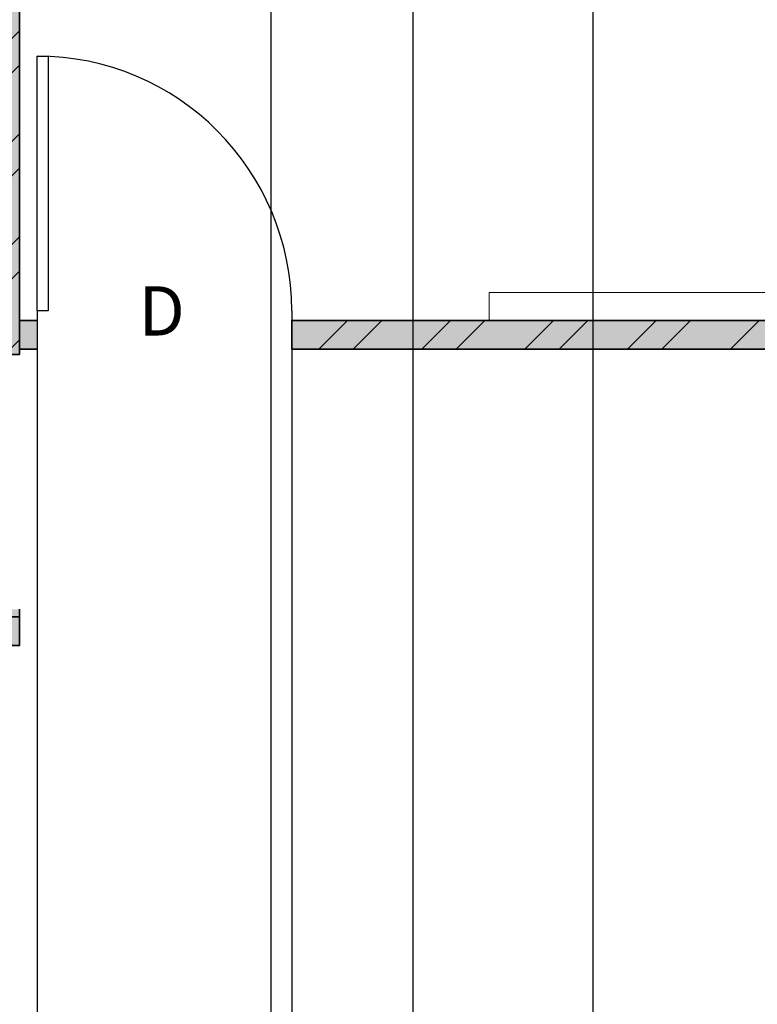
# Model space of a CAD drawing. Units: inches. Extents: x 1804 to 3296, y 909 to 2477.
# Tile 16 of 31: x 2119 to 2235, y 1484 to 1638. Entities that reach past the tile are written whole.
import ezdxf

# ---------------------------------------------------------------- set-up
doc = ezdxf.new("R2010")
doc.units = ezdxf.units.IN
for name, color, linetype, lineweight in [('A-ANNO-DIMS', 2, 'Continuous', 18), ('A-ANNO-TTLB', 156, 'Continuous', 35), ('A-WALL-PATT', 10, 'Continuous', 13), ('DOOR', 30, 'Continuous', 25), ('FUR', 100, 'Continuous', 18), ('TEXT', 190, 'Continuous', 18), ('WALL', 10, 'Continuous', 35)]:
    doc.layers.add(name, color=color, linetype=linetype, lineweight=lineweight)
doc.styles.get("Standard").update_dxf_attribs({"font": 'arial.ttf'})
doc.dimstyles.new('ISO-25', dxfattribs={"dimtxt": 5, "dimasz": 2.5, "dimexe": 1.25, "dimexo": 0.625, "dimtad": 1, "dimdec": 0, "dimlunit": 4, "dimtxsty": 'Standard', "dimcen": 2.5, "dimadec": 0, "dimazin": 0, "dimtfac": 1, "dimtdec": 0, "dimtmove": 0, "dimatfit": 3, "dimfxl": 1, "dimarcsym": 0})
pattern_1 = [(45, (0, 196.207), (-8.08223, 8.08223), []), (45, (5.388, 196.207), (-8.08223, 8.08223), [])]

# ---------------------------------------------------------------- blocks, each defined once
blk = doc.blocks.new('*U2')
for p, q in [((0, 0), (0, -6)), ((40, 0), (40, -6))]:
    blk.add_line(p, q)
blk.add_lwpolyline([(0, 0), (0, 40), (1.75, 40), (1.75, 0)], close=True)
blk.add_arc((0, 0), 40, 0, 90)
blk = doc.blocks.new('*D56')
at = {"layer": 'A-ANNO-DIMS', "color": 0, "lineweight": -2, "transparency": 16777216}
for p, q in [((2180.87, 1680.42), (2180.87, 975.89)), ((2268, 1680.42), (2268, 975.89)), ((2183.37, 977.14), (2265.5, 977.14))]:
    blk.add_line(p, q, dxfattribs=at)
at = {"layer": 'A-ANNO-DIMS', "color": 0, "lineweight": 100, "transparency": 16777216}
for points in [[(2183.37, 977.56), (2183.37, 976.72), (2180.87, 977.14)], [(2265.5, 977.56), (2265.5, 976.72), (2268, 977.14)]]:
    blk.add_solid(points, dxfattribs=at)
at = {"layer": 'Defpoints', "color": 0, "lineweight": 100, "transparency": 16777216}
for p in [(2180.87, 1681.04), (2268, 1681.04), (2268, 977.14)]:
    blk.add_point(p, dxfattribs=at)
at = {"layer": 'A-ANNO-DIMS', "color": 0, "transparency": 16777216, "insert": (2224.44, 980.32), "char_height": 5, "attachment_point": 5}
blk.add_mtext('7\'-3"', dxfattribs=at)
blk = doc.blocks.new('*D59')
at = {"layer": 'A-ANNO-DIMS', "color": 0, "lineweight": -2, "transparency": 16777216}
for p, q in [((2121.83, 1590.3), (2121.83, 975.89)), ((2161.83, 1590.3), (2161.83, 975.89)), ((2124.33, 977.14), (2159.33, 977.14))]:
    blk.add_line(p, q, dxfattribs=at)
at = {"layer": 'A-ANNO-DIMS', "color": 0, "lineweight": 100, "transparency": 16777216}
for points in [[(2124.33, 977.56), (2124.33, 976.72), (2121.83, 977.14)], [(2159.33, 977.56), (2159.33, 976.72), (2161.83, 977.14)]]:
    blk.add_solid(points, dxfattribs=at)
at = {"layer": 'Defpoints', "color": 0, "lineweight": 100, "transparency": 16777216}
for p in [(2121.83, 1590.92), (2161.83, 1590.92), (2161.83, 977.14)]:
    blk.add_point(p, dxfattribs=at)
at = {"layer": 'A-ANNO-DIMS', "color": 0, "transparency": 16777216, "insert": (2141.83, 980.32), "char_height": 5, "attachment_point": 5}
blk.add_mtext('3\'-4"', dxfattribs=at)
blk = doc.blocks.new('*D71')
at = {"layer": 'A-ANNO-DIMS', "color": 0, "lineweight": -2, "transparency": 16777216}
for p, q in [((2158.58, 1272.26), (2158.58, 1874.99)), ((2161.08, 1873.74), (2206.69, 1873.74)), ((2209.19, 1272.26), (2209.19, 1874.99))]:
    blk.add_line(p, q, dxfattribs=at)
at = {"layer": 'A-ANNO-DIMS', "color": 0, "lineweight": 100, "transparency": 16777216}
for points in [[(2161.08, 1874.15), (2161.08, 1873.32), (2158.58, 1873.74)], [(2206.69, 1874.15), (2206.69, 1873.32), (2209.19, 1873.74)]]:
    blk.add_solid(points, dxfattribs=at)
at = {"layer": 'Defpoints', "color": 0, "lineweight": 100, "transparency": 16777216}
for p in [(2209.19, 1873.74), (2158.58, 1271.63), (2209.19, 1271.63)]:
    blk.add_point(p, dxfattribs=at)
at = {"layer": 'A-ANNO-DIMS', "color": 0, "transparency": 16777216, "insert": (2183.88, 1876.95), "char_height": 5, "attachment_point": 5}
blk.add_mtext('4\'-2 1/2"', dxfattribs=at)

msp = doc.modelspace()

# ---------------------------------------------------------------- hatches: boundary and pattern name
at = {"layer": 'A-ANNO-TTLB'}
h = msp.add_hatch(color=256, dxfattribs=at)
h.dxf.hatch_style = 1
h.paths.add_polyline_path([(3294.53, 2476.54), (1803.79, 2476.54), (1805.43, 909.47), (3296.17, 909.47)])
h.paths.add_polyline_path([(1811, 914.33), (1812.79, 2467.54), (3285.53, 2467.54), (3283.74, 914.33)], flags=16)
h.paths.add_polyline_path([(1925.58, 1062.77), (1925.58, 1138.07), (1925.58, 1539.88), (1925.58, 1793.38), (1925.58, 1830.04), (2325.54, 1830.04), (2325.54, 1793.38), (2325.54, 1586.42), (2325.54, 1138.07), (2325.54, 1062.77)], flags=0)
h.paths.add_polyline_path([(1997.22, 1029.4), (2008.85, 1037.96), (2008.85, 1020.84)], flags=0)
h.paths.add_polyline_path([(1934.58, 1138.07), (1934.58, 1147.07), (2078.77, 1147.07), (2078.77, 1138.07), (2060.94, 1138.07)], flags=0)
h.paths.add_polyline_path([(1944.35, 1138.07), (1944.35, 1147.07), (2056.05, 1147.07), (2056.05, 1138.07)], flags=0)
h.paths.add_polyline_path([(2222.24, 1037.96), (2233.87, 1029.4), (2222.24, 1020.84)], flags=0)
h.paths.add_polyline_path([(2061.94, 1139.07), (2061.94, 1146.07), (2077.77, 1146.07), (2077.77, 1139.07)], flags=0)
h.paths.add_polyline_path([(2149.58, 1138.07), (2149.58, 1269.44), (2158.58, 1269.44), (2158.58, 1326.69), (2149.58, 1326.69), (2149.58, 1340.94), (2139.6, 1340.94), (2139.6, 1434.25), (2149.58, 1434.25), (2149.58, 1447.36), (2158.58, 1447.36), (2158.58, 1423.87), (2158.58, 1408.06), (2198.46, 1408.06), (2198.46, 1412.56), (2282.65, 1412.56), (2282.65, 1465.94), (2316.54, 1465.94), (2316.54, 1590.92), (2192.86, 1590.92), (2192.86, 1595.3), (2291.17, 1595.3), (2291.17, 1590.92), (2316.54, 1590.92), (2316.54, 1784.38), (2300.24, 1784.38), (2300.24, 1757.47), (2268, 1757.47), (2268, 1681.04), (2180.87, 1681.04), (2180.87, 1757.47), (2148.63, 1757.47), (2148.63, 1784.38), (2119.08, 1784.38), (2119.08, 1585.58), (2114.58, 1585.58), (2114.58, 1784.38), (2064.11, 1784.38), (2046.28, 1784.38), (2046.28, 1760.38), (1958.58, 1760.38), (1958.58, 1664.38), (1934.58, 1664.38), (1934.58, 1784.38), (1934.58, 1793.38), (2046.28, 1793.38), (2064.11, 1793.38), (2119.08, 1793.38), (2230.78, 1793.38), (2230.78, 1784.38), (2268, 1784.38), (2300.24, 1784.38), (2316.54, 1784.38), (2316.54, 1590.92), (2316.54, 1373.73), (2316.54, 1138.07)], flags=0)
h.paths.add_polyline_path([(2209.19, 1166.63), (2209.19, 1175.63), (2158.58, 1175.63), (2209.19, 1223.63), (2209.19, 1231.63), (2183.88, 1231.63), (2183.88, 1301.66), (2242.59, 1301.66), (2242.59, 1326.69), (2316.54, 1326.69), (2272.59, 1271.63), (2272.59, 1223.63), (2316.54, 1175.63), (2272.59, 1175.63), (2272.59, 1166.63)], flags=0)
h.paths.add_polyline_path([(1947.77, 1345.22), (1947.77, 1457.48), (1991.2, 1457.48), (1991.2, 1451.7), (1991.2, 1352.18), (1991.2, 1345.22)], flags=0)
h.paths.add_polyline_path([(2209.19, 1271.63), (2262.59, 1271.63), (2262.59, 1311.85), (2272.59, 1301.66), (2272.59, 1271.63), (2269.92, 1269.63), (2270.59, 1269.63), (2270.59, 1225.63), (2211.19, 1225.63), (2211.19, 1269.63), (2211.86, 1269.63)], flags=0)
h.paths.add_polyline_path([(2000.34, 1378.21), (2000.34, 1429.71), (2025.22, 1429.71), (2025.22, 1378.21)], flags=0)
h.paths.add_polyline_path([(2001.34, 1379.21), (2001.34, 1428.71), (2024.22, 1428.71), (2024.22, 1379.21)], flags=0)
h.paths.add_polyline_path([(2012.34, 1390.21), (2012.34, 1417.71), (2013.22, 1417.71), (2013.22, 1390.21)], flags=0)
h.paths.add_polyline_path([(2237.56, 1331.19), (2237.56, 1340.18), (2238.62, 1340.18), (2238.62, 1386.84), (2241.04, 1386.84), (2242.06, 1386.84), (2242.06, 1408.06), (2316.54, 1331.19)], flags=0)
h.paths.add_polyline_path([(1953.73, 1464.35), (1953.73, 1498.59), (1981.74, 1498.59), (1981.74, 1464.35)], flags=0)
h.paths.add_polyline_path([(1987.63, 1462.08), (1987.63, 1500.95), (2104.07, 1500.95), (2104.07, 1462.08), (2099.27, 1462.08), (1993.6, 1462.08)], flags=0)
h.paths.add_polyline_path([(1956.06, 1481.47, -1), (1979.41, 1481.47, -1)], flags=0)
edge = h.paths.add_edge_path(flags=0)
edge.add_ellipse((2299.53, 1438.37), major_axis=(0.31, 21.36), ratio=0.670333, start_angle=0, end_angle=360)
h.paths.add_polyline_path([(2297.39, 1438.37, -1), (2301.67, 1438.37, -1)], flags=0)
h.paths.add_polyline_path([(2591.54, 1163.23), (2591.54, 1179.38), (2591.54, 1379.68), (2591.54, 1395.84), (2734.5, 1395.84), (2734.5, 1379.68), (2734.5, 1179.38), (2734.5, 1163.23)], flags=0)
h.paths.add_polyline_path([(2592.54, 1164.23), (2592.54, 1166.23), (2733.5, 1166.23), (2733.5, 1164.23)], flags=0)
h.paths.add_polyline_path([(2592.54, 1180.38), (2592.54, 1378.68), (2733.5, 1378.68), (2733.5, 1180.38)], flags=0)
h.paths.add_polyline_path([(2593.54, 1181.38), (2593.54, 1377.68), (2732.5, 1377.68), (2732.5, 1181.38)], flags=0)
h.paths.add_polyline_path([(2594.54, 1182.38), (2594.54, 1376.68), (2731.5, 1376.68), (2731.5, 1182.38)], flags=0)
h.paths.add_polyline_path([(1936.95, 1697.46), (1936.95, 1736.46), (1955.41, 1736.46), (1955.41, 1697.46)], flags=0)
h.paths.add_polyline_path([(1938.48, 1718.36), (1938.48, 1734.92), (1953.65, 1734.92), (1953.65, 1718.36)], flags=0)
h.paths.add_polyline_path([(1944.75, 1726.64, -1), (1947.37, 1726.64, -1)], flags=0)
h.paths.add_polyline_path([(2592.54, 1394.84), (2733.5, 1394.84), (2733.5, 1392.84), (2592.54, 1392.84)], flags=0)
h.paths.add_polyline_path([(1976.61, 1762.5), (1976.61, 1781.44), (2012.79, 1781.44), (2012.79, 1762.5)], flags=0)
h.paths.add_polyline_path([(1979.57, 1771.97, -1), (1991.39, 1771.97, -1)], flags=0)
h.paths.add_polyline_path([(1995.36, 1771.97, -1), (2007.18, 1771.97, -1)], flags=0)
h.paths.add_polyline_path([(2251.51, 1744.53), (2268, 1730.05), (2251.51, 1730.05)], flags=0)
h.paths.add_polyline_path([(2047.28, 1785.38), (2047.28, 1792.38), (2063.11, 1792.38), (2063.11, 1785.38)], flags=0)
h.paths.add_polyline_path([(2155.08, 1770.92, -1), (2174.42, 1770.92, -1)], flags=0)
h.paths.add_polyline_path([(2188.59, 1758.27), (2188.59, 1772.81), (2222.3, 1772.81), (2222.3, 1758.27)], flags=0)
h.paths.add_polyline_path([(2223.97, 1758.27), (2223.97, 1772.81), (2257.68, 1772.81), (2257.68, 1758.27)], flags=0)
h.paths.add_polyline_path([(2274.45, 1770.92, -1), (2293.8, 1770.92, -1)], flags=0)
h.paths.add_polyline_path([(2591.54, 1582.09), (2591.54, 1782.39), (2734.5, 1782.39), (2734.5, 1582.09)], flags=0)
h.paths.add_polyline_path([(2592.54, 1583.09), (2592.54, 1781.39), (2733.5, 1781.39), (2733.5, 1583.09)], flags=0)
h.paths.add_polyline_path([(2593.54, 1584.09), (2593.54, 1780.39), (2732.5, 1780.39), (2732.5, 1584.09)], flags=0)
h.paths.add_polyline_path([(2594.54, 1585.09), (2594.54, 1779.39), (2731.5, 1779.39), (2731.5, 1585.09)], flags=0)
h.paths.add_polyline_path([(1922.17, 1978.79), (1922.17, 2295.08), (1922.17, 2296.08), (2115.67, 2296.08), (2115.67, 2384.31), (2115.67, 2385.31), (2322.12, 2385.31), (2323.12, 2385.31), (2323.12, 1979.79), (2323.12, 1978.79), (1923.17, 1978.79)], flags=0)
h.paths.add_polyline_path([(1922.17, 1978.79), (1922.17, 2051.31), (1922.17, 2214.86), (1922.17, 2296.08), (2115.67, 2296.08), (2115.67, 2385.31), (2323.12, 2385.31), (2323.12, 2280.42), (2323.12, 1978.79), (2115.67, 1978.79)], flags=0)
h.paths.add_polyline_path([(1923.17, 1979.79), (1923.17, 2050.31), (2115.67, 2050.31), (2115.67, 2051.31), (1923.17, 2051.31), (1923.17, 2213.86), (1923.17, 2214.86), (1923.17, 2295.08), (1990.02, 2295.08), (1990.02, 2214.86), (1991.02, 2214.86), (1991.02, 2295.08), (2115.67, 2295.08), (2115.67, 1979.79), (2116.67, 1979.79), (2116.67, 2304.18), (2116.67, 2384.31), (2322.12, 2384.31), (2322.12, 2280.42), (2322.12, 1979.79), (2115.67, 1979.79)], flags=0)
h.paths.add_polyline_path([(2972.46, 1192.5), (2972.46, 1196.92), (2995.47, 1196.92), (2995.47, 1255.47), (2995.09, 1255.47), (2987.42, 1249.39), (2980.08, 1255.47), (2978.05, 1255.47), (2978.05, 1257.24), (2995.47, 1257.24), (2995.47, 1261.58), (3015.37, 1261.58), (3015.37, 1333.28), (3015.37, 1414.4), (3032.82, 1414.4), (3032.82, 1333.28), (3032.82, 1261.58), (3052.66, 1261.58), (3052.66, 1255.47), (3079.86, 1255.47), (3078.72, 1254.57), (3081.47, 1252.29), (3078.56, 1249.99), (3075.81, 1252.26), (3072.57, 1249.69), (3070.36, 1251.52), (3067.67, 1249.39), (3060.34, 1255.47), (3052.66, 1255.47), (3052.66, 1196.92), (3054.58, 1196.92), (3074, 1196.92), (3074, 1192.5), (3052.66, 1192.5), (2995.47, 1192.5)], flags=0)
h.paths.add_polyline_path([(2490.75, 1979.27), (2490.75, 1980.27), (2596.87, 1980.27), (2596.87, 2051.8), (2596.87, 2052.8), (2596.87, 2216.35), (2596.87, 2297.57), (2717.32, 2297.57), (2710.57, 2305.62), (2724.07, 2305.62), (2717.32, 2297.57), (2782.37, 2297.57), (2782.37, 2395.8), (3006.82, 2395.8), (3006.82, 1981.27), (3093.73, 1981.27), (3093.73, 1980.27), (3047.51, 1980.27), (3046.37, 1979.37), (3049.11, 1977.1), (3046.2, 1974.79), (3043.46, 1977.07), (3040.21, 1974.49), (3038, 1976.32), (3035.32, 1974.2), (3027.98, 1980.27), (2871.83, 1980.27), (2871.83, 1981.27), (2791.37, 1981.27), (2791.37, 2050.8), (2597.87, 2050.8), (2597.87, 1980.27), (2597.87, 1979.27), (2546.27, 1979.27), (2545.12, 1978.37), (2547.87, 1976.1), (2544.96, 1973.79), (2542.22, 1976.07), (2538.97, 1973.49), (2536.76, 1975.32), (2534.07, 1973.2), (2526.74, 1979.27)], flags=0)
h.paths.add_polyline_path([(2597.87, 2051.8), (2606.87, 2051.8), (2606.87, 2258.39), (2597.87, 2258.39), (2597.87, 2296.57), (2606.87, 2296.57), (2606.87, 2262.39), (2782.37, 2262.39), (2782.37, 2296.57), (2790.37, 2296.57), (2790.37, 2262.39), (2791.37, 2262.39), (2791.37, 2305.67), (2791.37, 2385.8), (2996.82, 2385.8), (2996.82, 2339.85), (3006.82, 2339.85), (3006.82, 2250.12), (2997.82, 2250.12), (2997.82, 1981.27), (2996.82, 1981.27), (2872.83, 1981.27), (2872.83, 1991.8), (2871.83, 1991.8), (2871.83, 2050.8), (2790.37, 2050.8), (2597.87, 2050.8)], flags=0)
h.paths.add_polyline_path([(2179.93, 2153.92), (2179.93, 2353.97), (2259.98, 2353.97), (2259.98, 2153.92)], flags=0)
h.paths.add_polyline_path([(2180.93, 2154.92), (2180.93, 2352.97), (2258.98, 2352.97), (2258.98, 2154.92)], flags=0)
h.paths.add_polyline_path([(2960.87, 1608.49), (2960.87, 1753.62), (3070.9, 1753.62), (3070.9, 1608.49)], flags=0)
h.paths.add_polyline_path([(2961.87, 1609.49), (2961.87, 1752.62), (3069.9, 1752.62), (3069.9, 1609.49)], flags=0)
h.paths.add_polyline_path([(2962.87, 1610.49), (2962.87, 1751.62), (3068.9, 1751.62), (3068.9, 1610.49)], flags=0)
h.paths.add_polyline_path([(2963.87, 1611.49), (2963.87, 1750.62), (3067.9, 1750.62), (3067.9, 1611.49)], flags=0)
h.paths.add_polyline_path([(2782.37, 2051.8), (2782.37, 2216.32), (2791.37, 2216.32), (2791.37, 2051.8), (2872.83, 2051.8), (2872.83, 2068.56), (2884.67, 2068.56), (2884.67, 2085.33), (2896.51, 2085.33), (2896.51, 2102.09), (2908.36, 2102.09), (2908.36, 2118.85), (2920.2, 2118.85), (2920.2, 2135.62), (2932.05, 2135.62), (2932.05, 2145.3), (2925.08, 2145.3), (2925.08, 2203.2), (2996.82, 2203.2), (2996.82, 2145.3), (2953.82, 2145.3), (2872.83, 2051.8), (2790.37, 2051.8)], flags=0)
h.paths.add_polyline_path([(2717.32, 2238.65), (2710.57, 2246.7), (2724.07, 2246.7)], flags=0)
h.paths.add_polyline_path([(2003.09, 1122.79), (2017.16, 1122.79), (2017.16, 1138.74), (2003.09, 1138.74)], flags=8)
h.paths.add_polyline_path([(2174.76, 1792.72), (2188.83, 1792.72), (2188.83, 1808.66), (2174.76, 1808.66)], flags=8)
h.paths.add_polyline_path([(1987.95, 1792.51), (2002.02, 1792.51), (2002.02, 1808.45), (1987.95, 1808.45)], flags=8)
h.paths.add_polyline_path([(2148.79, 1289.26), (2160.46, 1289.26), (2160.46, 1305.2), (2148.79, 1305.2)], flags=8)
h.paths.add_polyline_path([(2115.36, 1133.57), (2127.04, 1133.57), (2127.04, 1149.51), (2115.36, 1149.51)], flags=8)
h.paths.add_polyline_path([(2237.58, 1421.48), (2249.25, 1421.48), (2249.25, 1437.43), (2237.58, 1437.43)], flags=8)
h.paths.add_polyline_path([(2134.99, 1584.32), (2146.66, 1584.32), (2146.66, 1600.26), (2134.99, 1600.26)], flags=8)
h.paths.add_polyline_path([(2101.95, 1557.31), (2113.62, 1557.31), (2113.62, 1573.25), (2101.95, 1573.25)], flags=8)
h.paths.add_polyline_path([(2937.85, 1156.77), (3120.41, 1156.77), (3120.41, 1185.72), (2937.85, 1185.72)], flags=8)
h.paths.add_polyline_path([(2980.71, 1786.71), (3050.06, 1786.71), (3050.06, 1802.66), (2980.71, 1802.66)], flags=8)
h.paths.add_polyline_path([(2869.28, 1661.96), (2938.62, 1661.96), (2938.62, 1690.8), (2869.28, 1690.8)], flags=8)
h.paths.add_polyline_path([(3092.27, 1674.86), (3161.62, 1674.86), (3161.62, 1690.8), (3092.27, 1690.8)], flags=8)
h.paths.add_polyline_path([(2980.71, 1674.86), (3050.06, 1674.86), (3050.06, 1690.8), (2980.71, 1690.8)], flags=8)
h.paths.add_polyline_path([(2649.07, 1678.23), (2674.53, 1678.23), (2674.53, 1714.76), (2649.07, 1714.76)], flags=8)
h.paths.add_polyline_path([(2530.84, 1981.63), (2549.13, 1981.63), (2549.13, 1997.57), (2530.84, 1997.57)], flags=8)
h.paths.add_polyline_path([(3031.29, 1981.77), (3049.58, 1981.77), (3049.58, 1997.71), (3031.29, 1997.71)], flags=8)
h.paths.add_polyline_path([(2715.38, 1911.9), (2851.54, 1911.9), (2851.54, 1940.85), (2715.38, 1940.85)], flags=8)
h.paths.add_polyline_path([(2015.23, 1927.36), (2205.42, 1927.36), (2205.42, 1956.3), (2015.23, 1956.3)], flags=8)
h.paths.add_polyline_path([(2671.84, 2057.84), (2702.75, 2057.84), (2702.75, 2073.79), (2671.84, 2073.79)], flags=8)
h.paths.add_polyline_path([(2678.5, 2316.52), (2765.26, 2316.52), (2765.26, 2332.46), (2678.5, 2332.46)], flags=8)
h.paths.add_polyline_path([(2678.48, 2271.96), (2736.41, 2271.96), (2736.41, 2287.9), (2678.48, 2287.9)], flags=8)
h.paths.add_polyline_path([(2019.2, 972.79), (2243.21, 972.79), (2243.21, 1001.74), (2019.2, 1001.74)], flags=8)
h.paths.add_polyline_path([(2097.06, 1021.56), (2132.16, 1021.56), (2132.16, 1037.51), (2097.06, 1037.51)], flags=8)
h.paths.add_polyline_path([(2182.47, 1360.48), (2207.35, 1360.48), (2207.35, 1376.42), (2182.47, 1376.42)], flags=8)
h.paths.add_polyline_path([(2261.12, 1361.77), (2295.01, 1361.77), (2295.01, 1377.71), (2261.12, 1377.71)], flags=8)
h.paths.add_polyline_path([(2245.75, 1511.51), (2278.44, 1511.51), (2278.44, 1527.46), (2245.75, 1527.46)], flags=8)
h.paths.add_polyline_path([(1991.16, 1296.29), (2060.51, 1296.29), (2060.51, 1312.23), (1991.16, 1312.23)], flags=8)
h.paths.add_polyline_path([(2187, 1651.35), (2246.71, 1651.35), (2246.71, 1667.29), (2187, 1667.29)], flags=8)
h.paths.add_polyline_path([(1976.49, 1684.81), (2068.63, 1684.81), (2068.63, 1700.76), (1976.49, 1700.76)], flags=8)
at = {"layer": 'A-WALL-PATT'}
h = msp.add_hatch(color=256, dxfattribs=at)
h.dxf.hatch_style = 1
h.paths.add_polyline_path([(2119.08, 1544.38), (1925.58, 1544.38), (1925.58, 1539.88), (2119.08, 1539.88)])
h.paths.add_polyline_path([(2119.08, 1545.58), (2114.58, 1545.58), (2114.58, 1544.38), (2119.08, 1544.38)])
h.paths.add_polyline_path([(1965.87, 1658.79), (1965.87, 1679.09), (1955.57, 1679.09), (1955.57, 1658.79)], flags=9)
h.paths.add_polyline_path([(2293.18, 1677.29), (2293.18, 1697.58), (2282.88, 1697.58), (2282.88, 1677.29)], flags=9)
h.paths.add_polyline_path([(2271.13, 1545.23), (2287.53, 1545.23), (2287.53, 1555.53), (2271.13, 1555.53)], flags=9)
h.paths.add_polyline_path([(2303.26, 1488.52), (2303.26, 1508.82), (2292.95, 1508.82), (2292.95, 1488.52)], flags=9)
h.paths.add_polyline_path([(2271.13, 1393.15), (2287.53, 1393.15), (2287.53, 1403.45), (2271.13, 1403.45)], flags=9)
h.paths.add_polyline_path([(2306.48, 1361.45), (2306.48, 1377.86), (2296.18, 1377.86), (2296.18, 1361.45)], flags=9)
h.paths.add_polyline_path([(2174.54, 1361.45), (2174.54, 1377.86), (2164.23, 1377.86), (2164.23, 1361.45)], flags=9)
h.paths.add_polyline_path([(1968.21, 1333.34), (1968.21, 1353.64), (1957.91, 1353.64), (1957.91, 1333.34)], flags=9)
h.paths.add_polyline_path([(2003.09, 1122.79), (2017.16, 1122.79), (2017.16, 1138.74), (2003.09, 1138.74)], flags=9)
h.paths.add_polyline_path([(2174.76, 1792.72), (2188.83, 1792.72), (2188.83, 1808.66), (2174.76, 1808.66)], flags=9)
h.paths.add_polyline_path([(1987.95, 1792.51), (2002.02, 1792.51), (2002.02, 1808.45), (1987.95, 1808.45)], flags=9)
h.paths.add_polyline_path([(2148.79, 1289.26), (2160.46, 1289.26), (2160.46, 1305.2), (2148.79, 1305.2)], flags=9)
h.paths.add_polyline_path([(2115.36, 1133.57), (2127.04, 1133.57), (2127.04, 1149.51), (2115.36, 1149.51)], flags=9)
h.paths.add_polyline_path([(2237.58, 1421.48), (2249.25, 1421.48), (2249.25, 1437.43), (2237.58, 1437.43)], flags=9)
h.paths.add_polyline_path([(2134.99, 1584.32), (2146.66, 1584.32), (2146.66, 1600.26), (2134.99, 1600.26)], flags=9)
h.paths.add_polyline_path([(2101.95, 1557.31), (2113.62, 1557.31), (2113.62, 1573.25), (2101.95, 1573.25)], flags=9)
h.paths.add_polyline_path([(2937.85, 1156.77), (3120.41, 1156.77), (3120.41, 1185.72), (2937.85, 1185.72)], flags=9)
h.paths.add_polyline_path([(2980.71, 1786.71), (3050.06, 1786.71), (3050.06, 1802.66), (2980.71, 1802.66)], flags=9)
h.paths.add_polyline_path([(2869.28, 1661.96), (2938.62, 1661.96), (2938.62, 1690.8), (2869.28, 1690.8)], flags=9)
h.paths.add_polyline_path([(3092.27, 1674.86), (3161.62, 1674.86), (3161.62, 1690.8), (3092.27, 1690.8)], flags=9)
h.paths.add_polyline_path([(2980.71, 1674.86), (3050.06, 1674.86), (3050.06, 1690.8), (2980.71, 1690.8)], flags=9)
h.paths.add_polyline_path([(2649.07, 1678.23), (2674.53, 1678.23), (2674.53, 1714.76), (2649.07, 1714.76)], flags=9)
h.paths.add_polyline_path([(2530.84, 1981.63), (2549.13, 1981.63), (2549.13, 1997.57), (2530.84, 1997.57)], flags=9)
h.paths.add_polyline_path([(3031.29, 1981.77), (3049.58, 1981.77), (3049.58, 1997.71), (3031.29, 1997.71)], flags=9)
h.paths.add_polyline_path([(2715.38, 1911.9), (2851.54, 1911.9), (2851.54, 1940.85), (2715.38, 1940.85)], flags=9)
h.paths.add_polyline_path([(2015.23, 1927.36), (2205.42, 1927.36), (2205.42, 1956.3), (2015.23, 1956.3)], flags=9)
h.paths.add_polyline_path([(2671.84, 2057.84), (2702.75, 2057.84), (2702.75, 2073.79), (2671.84, 2073.79)], flags=9)
h.paths.add_polyline_path([(2678.5, 2316.52), (2765.26, 2316.52), (2765.26, 2332.46), (2678.5, 2332.46)], flags=9)
h.paths.add_polyline_path([(2678.48, 2271.96), (2736.41, 2271.96), (2736.41, 2287.9), (2678.48, 2287.9)], flags=9)
h.paths.add_polyline_path([(2019.2, 972.79), (2243.21, 972.79), (2243.21, 1001.74), (2019.2, 1001.74)], flags=9)
h.paths.add_polyline_path([(2097.06, 1021.56), (2132.16, 1021.56), (2132.16, 1037.51), (2097.06, 1037.51)], flags=9)
h.paths.add_polyline_path([(2182.47, 1360.48), (2207.35, 1360.48), (2207.35, 1376.42), (2182.47, 1376.42)], flags=9)
h.paths.add_polyline_path([(2261.12, 1361.77), (2295.01, 1361.77), (2295.01, 1377.71), (2261.12, 1377.71)], flags=9)
h.paths.add_polyline_path([(2245.75, 1511.51), (2278.44, 1511.51), (2278.44, 1527.46), (2245.75, 1527.46)], flags=9)
h.paths.add_polyline_path([(1991.16, 1296.29), (2060.51, 1296.29), (2060.51, 1312.23), (1991.16, 1312.23)], flags=9)
h.paths.add_polyline_path([(2187, 1651.35), (2246.71, 1651.35), (2246.71, 1667.29), (2187, 1667.29)], flags=9)
h.paths.add_polyline_path([(1976.49, 1684.81), (2068.63, 1684.81), (2068.63, 1700.76), (1976.49, 1700.76)], flags=9)
h = msp.add_hatch(color=256, dxfattribs=at)
h.dxf.hatch_style = 1
h.paths.add_polyline_path([(2149.58, 1147.07), (2141.21, 1147.07), (2141.21, 1144.07), (2141.21, 1138.07), (2149.58, 1138.07)])
h.paths.add_polyline_path([(2101.21, 1144.07, -0.01877), (2101.32, 1147.07), (2078.77, 1147.07), (2078.77, 1138.07), (2101.21, 1138.07)])
h.paths.add_polyline_path([(2060.94, 1147.07), (2056.05, 1147.07), (2056.05, 1138.07), (2060.94, 1138.07)])
h.paths.add_polyline_path([(1944.35, 1147.07), (1934.58, 1147.07), (1934.58, 1138.07), (1944.35, 1138.07)])
h.paths.add_polyline_path([(2158.58, 1269.44), (2149.58, 1269.44), (2149.58, 1138.07), (2158.58, 1138.07)])
h.paths.add_polyline_path([(2003.09, 1122.79), (2017.16, 1122.79), (2017.16, 1138.74), (2003.09, 1138.74)], flags=9)
h.paths.add_polyline_path([(2174.76, 1792.72), (2188.83, 1792.72), (2188.83, 1808.66), (2174.76, 1808.66)], flags=9)
h.paths.add_polyline_path([(1987.95, 1792.51), (2002.02, 1792.51), (2002.02, 1808.45), (1987.95, 1808.45)], flags=9)
h.paths.add_polyline_path([(2148.79, 1289.26), (2160.46, 1289.26), (2160.46, 1305.2), (2148.79, 1305.2)], flags=9)
h.paths.add_polyline_path([(2115.36, 1133.57), (2127.04, 1133.57), (2127.04, 1149.51), (2115.36, 1149.51)], flags=9)
h.paths.add_polyline_path([(2237.58, 1421.48), (2249.25, 1421.48), (2249.25, 1437.43), (2237.58, 1437.43)], flags=9)
h.paths.add_polyline_path([(2134.99, 1584.32), (2146.66, 1584.32), (2146.66, 1600.26), (2134.99, 1600.26)], flags=9)
h.paths.add_polyline_path([(2101.95, 1557.31), (2113.62, 1557.31), (2113.62, 1573.25), (2101.95, 1573.25)], flags=9)
h.paths.add_polyline_path([(2937.85, 1156.77), (3120.41, 1156.77), (3120.41, 1185.72), (2937.85, 1185.72)], flags=9)
h.paths.add_polyline_path([(2980.71, 1786.71), (3050.06, 1786.71), (3050.06, 1802.66), (2980.71, 1802.66)], flags=9)
h.paths.add_polyline_path([(2869.28, 1661.96), (2938.62, 1661.96), (2938.62, 1690.8), (2869.28, 1690.8)], flags=9)
h.paths.add_polyline_path([(3092.27, 1674.86), (3161.62, 1674.86), (3161.62, 1690.8), (3092.27, 1690.8)], flags=9)
h.paths.add_polyline_path([(2980.71, 1674.86), (3050.06, 1674.86), (3050.06, 1690.8), (2980.71, 1690.8)], flags=9)
h.paths.add_polyline_path([(2649.07, 1678.23), (2674.53, 1678.23), (2674.53, 1714.76), (2649.07, 1714.76)], flags=9)
h.paths.add_polyline_path([(2530.84, 1981.63), (2549.13, 1981.63), (2549.13, 1997.57), (2530.84, 1997.57)], flags=9)
h.paths.add_polyline_path([(3031.29, 1981.77), (3049.58, 1981.77), (3049.58, 1997.71), (3031.29, 1997.71)], flags=9)
h.paths.add_polyline_path([(2715.38, 1911.9), (2851.54, 1911.9), (2851.54, 1940.85), (2715.38, 1940.85)], flags=9)
h.paths.add_polyline_path([(2015.23, 1927.36), (2205.42, 1927.36), (2205.42, 1956.3), (2015.23, 1956.3)], flags=9)
h.paths.add_polyline_path([(2671.84, 2057.84), (2702.75, 2057.84), (2702.75, 2073.79), (2671.84, 2073.79)], flags=9)
h.paths.add_polyline_path([(2678.5, 2316.52), (2765.26, 2316.52), (2765.26, 2332.46), (2678.5, 2332.46)], flags=9)
h.paths.add_polyline_path([(2678.48, 2271.96), (2736.41, 2271.96), (2736.41, 2287.9), (2678.48, 2287.9)], flags=9)
h.paths.add_polyline_path([(2019.2, 972.79), (2243.21, 972.79), (2243.21, 1001.74), (2019.2, 1001.74)], flags=9)
h.paths.add_polyline_path([(2097.06, 1021.56), (2132.16, 1021.56), (2132.16, 1037.51), (2097.06, 1037.51)], flags=9)
h.paths.add_polyline_path([(2182.47, 1360.48), (2207.35, 1360.48), (2207.35, 1376.42), (2182.47, 1376.42)], flags=9)
h.paths.add_polyline_path([(2261.12, 1361.77), (2295.01, 1361.77), (2295.01, 1377.71), (2261.12, 1377.71)], flags=9)
h.paths.add_polyline_path([(2245.75, 1511.51), (2278.44, 1511.51), (2278.44, 1527.46), (2245.75, 1527.46)], flags=9)
h.paths.add_polyline_path([(1991.16, 1296.29), (2060.51, 1296.29), (2060.51, 1312.23), (1991.16, 1312.23)], flags=9)
h.paths.add_polyline_path([(2187, 1651.35), (2246.71, 1651.35), (2246.71, 1667.29), (2187, 1667.29)], flags=9)
h.paths.add_polyline_path([(1976.49, 1684.81), (2068.63, 1684.81), (2068.63, 1700.76), (1976.49, 1700.76)], flags=9)
h = msp.add_hatch(color=256, dxfattribs=at)
h.dxf.hatch_style = 1
h.paths.add_polyline_path([(2158.58, 1275.49), (2155.29, 1275.49), (2149.58, 1275.49), (2149.58, 1269.44), (2158.58, 1269.44)])
h.paths.add_polyline_path([(2158.58, 1326.69), (2149.58, 1326.69), (2149.58, 1319.33), (2155.29, 1319.33), (2158.58, 1319.33)])
h.paths.add_polyline_path([(2158.58, 1402.2), (2158.58, 1423.87), (2158.58, 1447.36), (2149.58, 1447.36), (2149.58, 1423.87), (2149.58, 1340.94), (2149.58, 1326.69), (2158.58, 1326.69), (2158.58, 1354.23)])
h.paths.add_polyline_path([(1965.87, 1658.79), (1965.87, 1679.09), (1955.57, 1679.09), (1955.57, 1658.79)], flags=9)
h.paths.add_polyline_path([(2293.18, 1677.29), (2293.18, 1697.58), (2282.88, 1697.58), (2282.88, 1677.29)], flags=9)
h.paths.add_polyline_path([(2271.13, 1545.23), (2287.53, 1545.23), (2287.53, 1555.53), (2271.13, 1555.53)], flags=9)
h.paths.add_polyline_path([(2303.26, 1488.52), (2303.26, 1508.82), (2292.95, 1508.82), (2292.95, 1488.52)], flags=9)
h.paths.add_polyline_path([(2271.13, 1393.15), (2287.53, 1393.15), (2287.53, 1403.45), (2271.13, 1403.45)], flags=9)
h.paths.add_polyline_path([(2306.48, 1361.45), (2306.48, 1377.86), (2296.18, 1377.86), (2296.18, 1361.45)], flags=9)
h.paths.add_polyline_path([(2189.9, 1340.62), (2206.31, 1340.62), (2206.31, 1350.92), (2189.9, 1350.92)], flags=9)
h.paths.add_polyline_path([(2174.54, 1361.45), (2174.54, 1377.86), (2164.23, 1377.86), (2164.23, 1361.45)], flags=9)
h.paths.add_polyline_path([(2304.24, 1240.8), (2304.24, 1261.09), (2293.94, 1261.09), (2293.94, 1240.8)], flags=9)
h.paths.add_polyline_path([(2227.19, 1188.73), (2247.49, 1188.73), (2247.49, 1199.03), (2227.19, 1199.03)], flags=9)
h.paths.add_polyline_path([(2181.93, 1144.21), (2181.93, 1160.62), (2171.63, 1160.62), (2171.63, 1144.21)], flags=9)
h.paths.add_polyline_path([(1968.21, 1333.34), (1968.21, 1353.64), (1957.91, 1353.64), (1957.91, 1333.34)], flags=9)
h.paths.add_polyline_path([(2029.78, 1203.53), (2053.95, 1203.53), (2053.95, 1213.83), (2029.78, 1213.83)], flags=9)
h.paths.add_polyline_path([(2576.51, 1671.88), (2576.51, 1692.17), (2566.21, 1692.17), (2566.21, 1671.88)], flags=9)
h.paths.add_polyline_path([(2566.99, 1269.67), (2566.99, 1289.96), (2556.68, 1289.96), (2556.68, 1269.67)], flags=9)
h.paths.add_polyline_path([(2581.85, 1269.17), (2581.85, 1289.46), (2571.54, 1289.46), (2571.54, 1269.17)], flags=9)
h.paths.add_polyline_path([(2650.71, 1409.75), (2674.89, 1409.75), (2674.89, 1420.05), (2650.71, 1420.05)], flags=9)
h.paths.add_polyline_path([(2003.09, 1122.79), (2017.16, 1122.79), (2017.16, 1138.74), (2003.09, 1138.74)], flags=9)
h.paths.add_polyline_path([(2174.76, 1792.72), (2188.83, 1792.72), (2188.83, 1808.66), (2174.76, 1808.66)], flags=9)
h.paths.add_polyline_path([(1987.95, 1792.51), (2002.02, 1792.51), (2002.02, 1808.45), (1987.95, 1808.45)], flags=9)
h.paths.add_polyline_path([(2148.79, 1289.26), (2160.46, 1289.26), (2160.46, 1305.2), (2148.79, 1305.2)], flags=9)
h.paths.add_polyline_path([(2115.36, 1133.57), (2127.04, 1133.57), (2127.04, 1149.51), (2115.36, 1149.51)], flags=9)
h.paths.add_polyline_path([(2237.58, 1421.48), (2249.25, 1421.48), (2249.25, 1437.43), (2237.58, 1437.43)], flags=9)
h.paths.add_polyline_path([(2134.99, 1584.32), (2146.66, 1584.32), (2146.66, 1600.26), (2134.99, 1600.26)], flags=9)
h.paths.add_polyline_path([(2101.95, 1557.31), (2113.62, 1557.31), (2113.62, 1573.25), (2101.95, 1573.25)], flags=9)
h.paths.add_polyline_path([(2937.85, 1156.77), (3120.41, 1156.77), (3120.41, 1185.72), (2937.85, 1185.72)], flags=9)
h.paths.add_polyline_path([(2980.71, 1786.71), (3050.06, 1786.71), (3050.06, 1802.66), (2980.71, 1802.66)], flags=9)
h.paths.add_polyline_path([(2869.28, 1661.96), (2938.62, 1661.96), (2938.62, 1690.8), (2869.28, 1690.8)], flags=9)
h.paths.add_polyline_path([(3092.27, 1674.86), (3161.62, 1674.86), (3161.62, 1690.8), (3092.27, 1690.8)], flags=9)
h.paths.add_polyline_path([(2980.71, 1674.86), (3050.06, 1674.86), (3050.06, 1690.8), (2980.71, 1690.8)], flags=9)
h.paths.add_polyline_path([(2649.07, 1678.23), (2674.53, 1678.23), (2674.53, 1714.76), (2649.07, 1714.76)], flags=9)
h.paths.add_polyline_path([(2530.84, 1981.63), (2549.13, 1981.63), (2549.13, 1997.57), (2530.84, 1997.57)], flags=9)
h.paths.add_polyline_path([(3031.29, 1981.77), (3049.58, 1981.77), (3049.58, 1997.71), (3031.29, 1997.71)], flags=9)
h.paths.add_polyline_path([(2715.38, 1911.9), (2851.54, 1911.9), (2851.54, 1940.85), (2715.38, 1940.85)], flags=9)
h.paths.add_polyline_path([(2015.23, 1927.36), (2205.42, 1927.36), (2205.42, 1956.3), (2015.23, 1956.3)], flags=9)
h.paths.add_polyline_path([(2671.84, 2057.84), (2702.75, 2057.84), (2702.75, 2073.79), (2671.84, 2073.79)], flags=9)
h.paths.add_polyline_path([(2678.5, 2316.52), (2765.26, 2316.52), (2765.26, 2332.46), (2678.5, 2332.46)], flags=9)
h.paths.add_polyline_path([(2678.48, 2271.96), (2736.41, 2271.96), (2736.41, 2287.9), (2678.48, 2287.9)], flags=9)
h.paths.add_polyline_path([(2019.2, 972.79), (2243.21, 972.79), (2243.21, 1001.74), (2019.2, 1001.74)], flags=9)
h.paths.add_polyline_path([(2097.06, 1021.56), (2132.16, 1021.56), (2132.16, 1037.51), (2097.06, 1037.51)], flags=9)
h.paths.add_polyline_path([(2182.47, 1360.48), (2207.35, 1360.48), (2207.35, 1376.42), (2182.47, 1376.42)], flags=9)
h.paths.add_polyline_path([(2261.12, 1361.77), (2295.01, 1361.77), (2295.01, 1377.71), (2261.12, 1377.71)], flags=9)
h.paths.add_polyline_path([(2245.75, 1511.51), (2278.44, 1511.51), (2278.44, 1527.46), (2245.75, 1527.46)], flags=9)
h.paths.add_polyline_path([(1991.16, 1296.29), (2060.51, 1296.29), (2060.51, 1312.23), (1991.16, 1312.23)], flags=9)
h.paths.add_polyline_path([(2187, 1651.35), (2246.71, 1651.35), (2246.71, 1667.29), (2187, 1667.29)], flags=9)
h.paths.add_polyline_path([(1976.49, 1684.81), (2068.63, 1684.81), (2068.63, 1700.76), (1976.49, 1700.76)], flags=9)
h = msp.add_hatch(dxfattribs=at)
h.set_pattern_fill('ANSI32', color=256, scale=1.2)
h.set_pattern_definition(pattern_1)
h.paths.add_polyline_path([(1934.58, 1784.38), (1934.58, 1793.38), (1925.58, 1793.38), (1925.58, 1539.88), (2119.08, 1539.88), (2119.08, 1545.58), (2114.58, 1545.58), (2114.58, 1544.38), (1934.58, 1544.38)])
h.paths.add_polyline_path([(2114.58, 1793.38), (2064.11, 1793.38), (2064.11, 1784.38), (2114.58, 1784.38)], flags=17)
h.paths.add_polyline_path([(2325.54, 1793.38), (2230.78, 1793.38), (2230.78, 1784.38), (2268, 1784.38), (2300.24, 1784.38), (2316.54, 1784.38), (2316.54, 1590.92), (2316.54, 1586.42), (2325.54, 1586.42)])
h.paths.add_polyline_path([(1944.35, 1147.07), (1934.58, 1147.07), (1934.58, 1138.07), (1944.35, 1138.07)])
h.paths.add_polyline_path([(2101.21, 1144.07, -0.01877), (2101.32, 1147.07), (2078.77, 1147.07), (2078.77, 1138.07), (2101.21, 1138.07)])
h.paths.add_polyline_path([(1934.58, 1539.88), (1925.58, 1539.88), (1925.58, 1138.07), (1934.58, 1138.07), (1934.58, 1147.07)])
h.paths.add_polyline_path([(2325.54, 1586.42), (2316.54, 1586.42), (2316.54, 1373.73), (2316.54, 1138.07), (2325.54, 1138.07), (2325.54, 1228.97)])
h.paths.add_polyline_path([(2158.58, 1423.87), (2158.58, 1447.36), (2149.58, 1447.36), (2149.58, 1423.87), (2149.58, 1340.94), (2149.58, 1326.69), (2158.58, 1326.69), (2158.58, 1354.23), (2158.58, 1402.2)])
h.paths.add_polyline_path([(2316.54, 1412.56), (2282.65, 1412.56), (2273.09, 1412.56), (2273.09, 1408.06), (2316.54, 1408.06)])
h.paths.add_polyline_path([(2273.09, 1412.56), (2242.06, 1412.56), (2242.06, 1408.06), (2273.09, 1408.06)])
h.paths.add_polyline_path([(2237.56, 1412.56), (2198.46, 1412.56), (2198.46, 1408.06), (2237.56, 1408.06)])
h.paths.add_polyline_path([(2242.06, 1408.06), (2237.56, 1408.06), (2237.56, 1386.84), (2242.06, 1386.84)])
h.paths.add_polyline_path([(2242.06, 1412.56), (2237.56, 1412.56), (2237.56, 1408.06), (2242.06, 1408.06)])
h.paths.add_polyline_path([(2158.58, 1269.44), (2149.58, 1269.44), (2149.58, 1138.07), (2158.58, 1138.07)])
h.paths.add_polyline_path([(2149.58, 1147.07), (2141.21, 1147.07), (2141.21, 1144.07), (2141.21, 1138.07), (2149.58, 1138.07)])
h.paths.add_polyline_path([(2272.59, 1175.63), (2209.19, 1175.63), (2209.19, 1166.63), (2272.59, 1166.63)])
h.paths.add_polyline_path([(2237.56, 1446.21), (2242.06, 1446.21), (2242.06, 1586.42), (2237.56, 1586.42)])
h.paths.add_polyline_path([(2242.06, 1414.58), (2237.56, 1414.58), (2237.56, 1412.56), (2242.06, 1412.56)])
h = msp.add_hatch(color=256, dxfattribs=at)
h.dxf.hatch_style = 1
h.paths.add_polyline_path([(2114.58, 1793.38), (2064.11, 1793.38), (2064.11, 1784.38), (2114.58, 1784.38)])
h.paths.add_polyline_path([(2119.08, 1793.38), (2114.58, 1793.38), (2114.58, 1585.58), (2119.08, 1585.58)])
h.paths.add_polyline_path([(2325.54, 1793.38), (2230.78, 1793.38), (2230.78, 1784.38), (2268, 1784.38), (2316.54, 1784.38), (2316.54, 1590.92), (2316.54, 1586.42), (2325.54, 1586.42)])
h.paths.add_polyline_path([(2316.54, 1331.19), (2158.58, 1331.19), (2158.58, 1326.69), (2316.54, 1326.69)])
h.paths.add_polyline_path([(2242.06, 1408.06), (2237.56, 1408.06), (2237.56, 1386.84), (2242.06, 1386.84)])
h.paths.add_polyline_path([(2242.06, 1412.56), (2237.56, 1412.56), (2237.56, 1408.06), (2242.06, 1408.06)])
h.paths.add_polyline_path([(2237.56, 1412.56), (2198.46, 1412.56), (2198.46, 1408.06), (2237.56, 1408.06)])
h.paths.add_polyline_path([(2273.09, 1412.56), (2242.06, 1412.56), (2242.06, 1408.06), (2273.09, 1408.06)])
h.paths.add_polyline_path([(2316.54, 1412.56), (2282.65, 1412.56), (2273.09, 1412.56), (2273.09, 1408.06), (2316.54, 1408.06)])
h.paths.add_polyline_path([(2325.54, 1586.42), (2316.54, 1586.42), (2316.54, 1373.73), (2316.54, 1138.07), (2325.54, 1138.07), (2325.54, 1228.97)])
h.paths.add_polyline_path([(2272.59, 1175.63), (2209.19, 1175.63), (2209.19, 1166.63), (2272.59, 1166.63)])
h = msp.add_hatch(dxfattribs=at)
h.set_pattern_fill('ANSI32', color=256, scale=1.2)
h.set_pattern_definition(pattern_1)
h.paths.add_polyline_path([(2114.58, 1585.58), (2119.08, 1585.58), (2119.08, 1793.38), (2114.58, 1793.38)])
h = msp.add_hatch(color=256, dxfattribs=at)
h.dxf.hatch_style = 1
h.paths.add_polyline_path([(2121.83, 1590.92), (2119.08, 1590.92), (2119.08, 1586.42), (2121.83, 1586.42)])
h = msp.add_hatch(dxfattribs=at)
h.set_pattern_fill('ANSI32', color=256, scale=1.2)
h.set_pattern_definition(pattern_1)
h.paths.add_polyline_path([(2161.83, 1590.92), (2161.83, 1586.42), (2316.54, 1586.42), (2316.54, 1590.92)])
h = msp.add_hatch(color=256, dxfattribs=at)
h.dxf.hatch_style = 1
h.paths.add_polyline_path([(2316.54, 1590.92), (2161.83, 1590.92), (2161.83, 1586.42), (2316.54, 1586.42)])

# ---------------------------------------------------------------- linework, layer by layer
at = {"layer": 'FUR'}
msp.add_lwpolyline([(2192.86, 1590.92), (2291.17, 1590.92), (2291.17, 1595.3), (2192.86, 1595.3)], close=True, dxfattribs=at)
at = {"layer": 'WALL'}
for p, q in [((2119.08, 1793.38), (2119.08, 1585.58)), ((2121.83, 1590.92), (2119.08, 1590.92)), ((2316.54, 1590.92), (2161.83, 1590.92)), ((2121.83, 1586.42), (2119.08, 1586.42)), ((2325.54, 1586.42), (2161.83, 1586.42)), ((2119.08, 1545.58), (2119.08, 1539.88)), ((2119.08, 1539.88), (1925.58, 1539.88))]:
    msp.add_line(p, q, dxfattribs=at)
for points in [[(2114.58, 1585.58), (2119.08, 1585.58), (2119.08, 1793.38), (2114.58, 1793.38)], [(2161.83, 1586.42), (2316.54, 1586.42), (2316.54, 1590.92), (2161.83, 1590.92)], [(1925.58, 1539.88), (2119.08, 1539.88), (2119.08, 1544.38), (1925.58, 1544.38)]]:
    msp.add_lwpolyline(points, close=True, dxfattribs=at)

# ---------------------------------------------------------------- block references
at = {"layer": 'DOOR'}
msp.add_blockref('*U2', (2121.83, 1592.42), dxfattribs=at)

# ---------------------------------------------------------------- texts
at = {"layer": 'TEXT', "insert": (2137.76, 1596.28), "char_height": 7.74, "attachment_point": 1}
msp.add_mtext_dynamic_manual_height_columns('D', width=163.3261, gutter_width=38.69, heights=[0], dxfattribs=at)

# ---------------------------------------------------------------- dimensions: what is measured, and where the dimension line sits
at = {"layer": 'A-ANNO-DIMS'}
for base, p1, p2, picture, middle in [((2209.19, 1873.74), (2158.58, 1271.63), (2209.19, 1271.63), '*D71', (2183.88, 1876.95)), ((2268, 977.14), (2180.87, 1681.04), (2268, 1681.04), '*D56', (2224.44, 980.32)), ((2161.83, 977.14), (2121.83, 1590.92), (2161.83, 1590.92), '*D59', (2141.83, 980.32))]:
    dim = msp.add_linear_dim(base=base, p1=p1, p2=p2, dimstyle='ISO-25', override={"dimdec": 1, "dimlfac": 1, "dimrnd": 0, "dimzin": 1, "dimdsep": 46, "dimlunit": 4, "dimfrac": 2}, dxfattribs=at)
    dim.commit()
    dim.dimension.update_dxf_attribs({"geometry": picture, "text_midpoint": middle})

doc.saveas('drawing.dxf')
